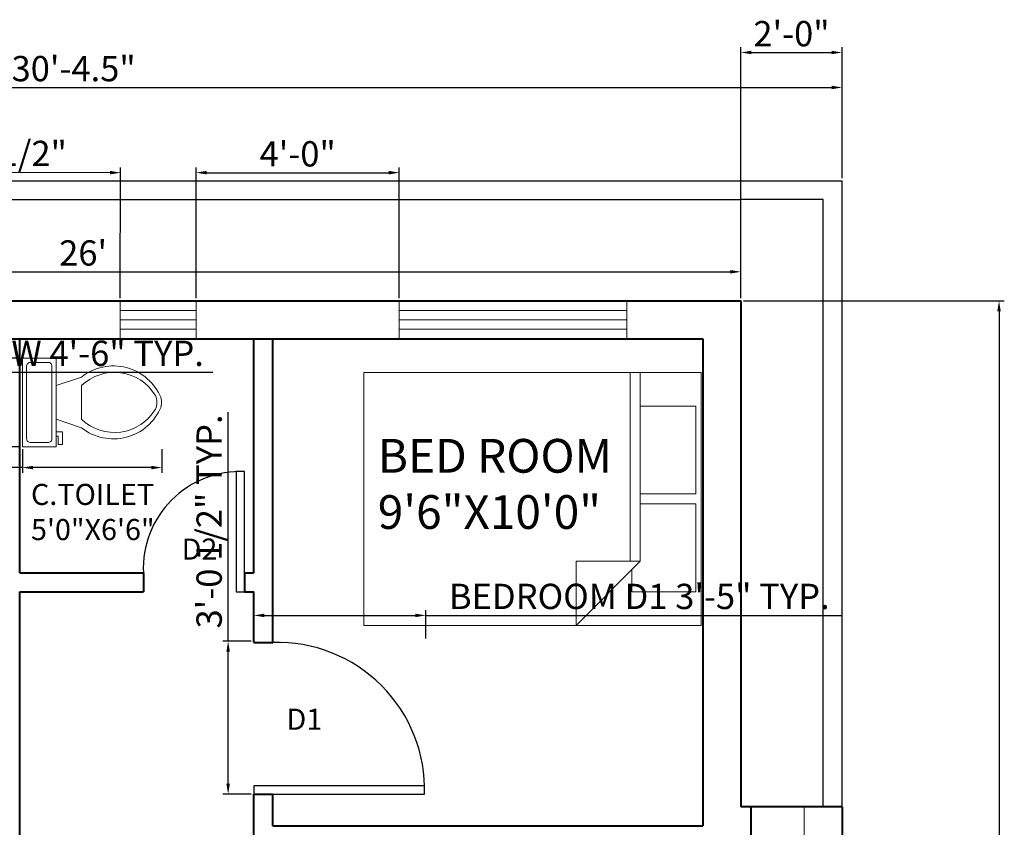
# Model space of a CAD drawing. Units: inches. Extents: x 459864 to 460310, y 324185 to 324787.
# Tile 112 of 112: x 460076 to 460310, y 324591 to 324782. Entities that reach past the tile are written whole.
import ezdxf

# ---------------------------------------------------------------- set-up
doc = ezdxf.new("R2010")
doc.units = ezdxf.units.IN
doc.linetypes.add('ACAD_ISO02W100', pattern=[15, 12, -3])
for name, color, linetype, lineweight in [('A-ANNO-DIMS', 2, 'Continuous', 18), ('A-ANNO-TEXT', 7, 'Continuous', 18), ('A-AREA-IDEN', 7, 'Continuous', 25), ('A-DOOR', 3, 'Continuous', 25), ('A-FLOR-FIXT', 9, 'Continuous', 18), ('A-FURN', 8, 'Continuous', 18), ('A-GLAZ', 4, 'Continuous', 18), ('A-WALL', 7, 'Continuous', 40), ('A-WALL-OVHD', 7, 'ACAD_ISO02W100', 18), ('C-PROP', 7, 'Continuous', 30)]:
    doc.layers.add(name, color=color, linetype=linetype, lineweight=lineweight)
doc.styles.get("Standard").update_dxf_attribs({"font": 'arial.ttf'})
doc.dimstyles.new('ISO-25', dxfattribs={"dimtxt": 6, "dimasz": 2.5, "dimexe": 1.25, "dimexo": 0.625, "dimtad": 1, "dimdec": 1, "dimlunit": 3, "dimtxsty": 'Standard', "dimcen": 2.5, "dimadec": 0, "dimazin": 0, "dimtfac": 1, "dimtdec": 1, "dimtmove": 0, "dimatfit": 3, "dimfxl": 1, "dimarcsym": 0})

# ---------------------------------------------------------------- blocks, each defined once
blk = doc.blocks.new('Window - Wood Frame 36 in. Wide plan')
for p, q in [((0, 6), (0, 0)), ((36, 6), (36, 0)), ((0, 4.5), (36, 4.5)), ((0, 3), (36, 3)), ((0, 1.5), (36, 1.5))]:
    blk.add_line(p, q)
blk = doc.blocks.new('Toilet - top')
for p, q in [((9.5, -6), (9.5, -2)), ((-10, -8.5), (-8, -8.5)), ((-10, -9.5), (-10, -8.5)), ((-8, -8.5), (-8, -8)), ((-7, -8), (-7, -9.5)), ((-4, -8), (-6, -14)), ((4, -8), (6, -14)), ((-7, -9.5), (-10, -9.5)), ((4, -14), (-4, -14))]:
    blk.add_line(p, q)
blk.add_lwpolyline([(10.5, -8), (10.5, 0), (-10.5, 0), (-10.5, -8)], close=True)
for points in [[(-9.5, -2), (-9.5, -6)], [(8.5, -1), (-8.5, -1)], [(-8.5, -7), (8.5, -7)]]:
    blk.add_lwpolyline(points)
for centre, radius, start, end in [((-8.62, -1.88), 0.884, 81.8699, 188.1301), ((8.62, -1.88), 0.884, 351.8699, 98.1301), ((-8.62, -6.12), 0.884, 171.8699, 278.1301), ((8.62, -6.12), 0.884, 261.8699, 8.1301), ((3.52, -21.58), 12.17, 141.4691, 247.9714), ((4.2, -21.82), 11.33, 136.3677, 238.9468), ((-3.52, -21.58), 12.17, 292.0284, 38.5307), ((-4.2, -21.82), 11.33, 301.053, 43.6321), ((0, -27.88), 4, 245.7318, 294.2682), ((0, -29), 4, 254.8605, 285.1395)]:
    blk.add_arc(centre, radius, start, end)
blk = doc.blocks.new('Bed - Queen')
for p, q in [((0, -80.00003), (0, 0)), ((0, 0), (59.99999, 0)), ((59.99999, 0), (59.99999, -80.00003)), ((7.99999, -1.2), (28.79998, -1.2)), ((7.99999, -14.4), (7.99999, -1.2)), ((28.79998, -1.2), (28.79998, -14.4)), ((31.19999, -1.2), (51.99999, -1.2)), ((31.19999, -14.4), (31.19999, -1.2)), ((51.99999, -1.2), (51.99999, -16.4)), ((0, -14.4), (44.8, -14.4)), ((59.99999, -29.6), (44.8, -14.4)), ((44.8, -14.4), (44.8, -29.6)), ((44.8, -16.8), (0, -16.8)), ((51.99999, -16.4), (46.79936, -16.4)), ((44.8, -29.6), (59.99999, -29.6)), ((59.99999, -80.00003), (0, -80.00003))]:
    blk.add_line(p, q)
blk = doc.blocks.new('*D19')
at = {"layer": 'A-ANNO-DIMS', "color": 0, "lineweight": -2, "transparency": 16777216}
for p, q in [((459935.11, 324716.11), (459935.11, 324723.62)), ((459937.61, 324722.37), (460244.61, 324722.37)), ((460247.11, 324716.11), (460247.11, 324723.62))]:
    blk.add_line(p, q, dxfattribs=at)
at = {"layer": 'A-ANNO-DIMS', "color": 0, "transparency": 16777216}
for points in [[(459937.61, 324722.79), (459937.61, 324721.96), (459935.11, 324722.37)], [(460244.61, 324722.79), (460244.61, 324721.96), (460247.11, 324722.37)]]:
    blk.add_solid(points, dxfattribs=at)
at = {"layer": 'Defpoints', "color": 0, "transparency": 16777216}
for p in [(460247.11, 324722.37), (459935.11, 324715.48), (460247.11, 324715.48)]:
    blk.add_point(p, dxfattribs=at)
at = {"layer": 'A-ANNO-DIMS', "color": 0, "transparency": 16777216, "insert": (460091.11, 324726.06), "char_height": 6, "attachment_point": 5}
blk.add_mtext("26'", dxfattribs=at)
blk = doc.blocks.new('*D20')
at = {"layer": 'A-ANNO-DIMS', "color": 0, "lineweight": -2, "transparency": 16777216}
for p, q in [((459906.61, 324744.61), (459906.61, 324767.34)), ((459909.11, 324766.09), (460268.61, 324766.09)), ((460271.11, 324744.61), (460271.11, 324767.34))]:
    blk.add_line(p, q, dxfattribs=at)
at = {"layer": 'A-ANNO-DIMS', "color": 0, "transparency": 16777216}
for points in [[(459909.11, 324766.5), (459909.11, 324765.67), (459906.61, 324766.09)], [(460268.61, 324766.5), (460268.61, 324765.67), (460271.11, 324766.09)]]:
    blk.add_solid(points, dxfattribs=at)
at = {"layer": 'Defpoints', "color": 0, "transparency": 16777216}
for p in [(460271.11, 324766.09), (459906.61, 324743.98), (460271.11, 324743.98)]:
    blk.add_point(p, dxfattribs=at)
at = {"layer": 'A-ANNO-DIMS', "color": 0, "transparency": 16777216, "insert": (460088.86, 324769.78), "char_height": 6, "attachment_point": 5}
blk.add_mtext('30\'-4.5"', dxfattribs=at)
blk = doc.blocks.new('*D21')
at = {"layer": 'A-ANNO-DIMS', "color": 0, "lineweight": -2, "transparency": 16777216}
for p, q in [((460247.74, 324715.48), (460309.58, 324715.48)), ((460308.33, 324712.98), (460308.33, 324285.98)), ((460247.74, 324283.48), (460309.58, 324283.48))]:
    blk.add_line(p, q, dxfattribs=at)
at = {"layer": 'A-ANNO-DIMS', "color": 0, "transparency": 16777216}
for points in [[(460307.91, 324712.98), (460308.75, 324712.98), (460308.33, 324715.48)], [(460307.91, 324285.98), (460308.75, 324285.98), (460308.33, 324283.48)]]:
    blk.add_solid(points, dxfattribs=at)
at = {"layer": 'Defpoints', "color": 0, "transparency": 16777216}
for p in [(460247.11, 324715.48), (460247.11, 324283.48), (460308.33, 324283.48)]:
    blk.add_point(p, dxfattribs=at)
at = {"layer": 'A-ANNO-DIMS', "color": 0, "transparency": 16777216, "insert": (460304.64, 324499.48), "char_height": 6, "attachment_point": 5, "rotation": 90}
blk.add_mtext("36'", dxfattribs=at)
blk = doc.blocks.new('DOOR-SWING-36IN')
for p, q in [((40.5, 2), (0, 2)), ((0, 2), (0, 0)), ((40.5, 0), (40.5, 2)), ((4.5, 0), (40.5, 0))]:
    blk.add_line(p, q)
blk.add_arc((5.5, 1), 35.01, 358.3634, 91.6366)
blk = doc.blocks.new('*D24')
at = {"layer": 'A-ANNO-DIMS', "color": 0, "lineweight": -2, "transparency": 16777216}
for p, q in [((459988.23, 324706.02), (459988.23, 324697.29)), ((460042.23, 324706.02), (460042.23, 324697.29)), ((459990.73, 324698.54), (460039.73, 324698.54)), ((460042.23, 324698.54), (460121.9, 324698.54))]:
    blk.add_line(p, q, dxfattribs=at)
at = {"layer": 'A-ANNO-DIMS', "color": 0, "transparency": 16777216}
for points in [[(459990.73, 324698.96), (459990.73, 324698.13), (459988.23, 324698.54)], [(460039.73, 324698.96), (460039.73, 324698.13), (460042.23, 324698.54)]]:
    blk.add_solid(points, dxfattribs=at)
at = {"layer": 'Defpoints', "color": 0, "transparency": 16777216}
for p in [(459988.23, 324706.64), (460042.23, 324706.64), (460042.23, 324698.54)]:
    blk.add_point(p, dxfattribs=at)
at = {"layer": 'A-ANNO-DIMS', "color": 0, "transparency": 16777216, "insert": (460083.32, 324702.27), "char_height": 6, "attachment_point": 5}
blk.add_mtext('WINDOW 4\'-6" TYP.', dxfattribs=at)
blk = doc.blocks.new('*D30')
at = {"layer": 'A-ANNO-DIMS', "color": 0, "lineweight": -2, "transparency": 16777216}
for p, q in [((460076.72, 324680.27), (460076.72, 324674.69)), ((460109.77, 324680.27), (460109.77, 324674.69)), ((460076.72, 324675.94), (460019.86, 324675.94)), ((460107.27, 324675.94), (460079.22, 324675.94))]:
    blk.add_line(p, q, dxfattribs=at)
at = {"layer": 'A-ANNO-DIMS', "color": 0, "transparency": 16777216}
for points in [[(460079.22, 324676.36), (460079.22, 324675.52), (460076.72, 324675.94)], [(460107.27, 324676.36), (460107.27, 324675.52), (460109.77, 324675.94)]]:
    blk.add_solid(points, dxfattribs=at)
at = {"layer": 'Defpoints', "color": 0, "transparency": 16777216}
for p in [(460076.72, 324680.9), (460109.77, 324680.9), (460076.72, 324675.94)]:
    blk.add_point(p, dxfattribs=at)
at = {"layer": 'A-ANNO-DIMS', "color": 0, "transparency": 16777216, "insert": (460047.04, 324679.67), "char_height": 6, "attachment_point": 5}
blk.add_mtext('WC 2\'-9" TYP.', dxfattribs=at)
blk = doc.blocks.new('*D31')
at = {"layer": 'A-ANNO-DIMS', "color": 0, "lineweight": -2, "transparency": 16777216}
for p, q in [((460071.76, 324701.9), (460071.76, 324741.66)), ((460076.09, 324701.9), (460070.51, 324701.9)), ((460071.76, 324683.4), (460071.76, 324699.4)), ((460076.09, 324680.9), (460070.51, 324680.9))]:
    blk.add_line(p, q, dxfattribs=at)
at = {"layer": 'A-ANNO-DIMS', "color": 0, "transparency": 16777216}
for points in [[(460071.35, 324699.4), (460072.18, 324699.4), (460071.76, 324701.9)], [(460071.35, 324683.4), (460072.18, 324683.4), (460071.76, 324680.9)]]:
    blk.add_solid(points, dxfattribs=at)
at = {"layer": 'Defpoints', "color": 0, "transparency": 16777216}
for p in [(460071.76, 324701.9), (460076.72, 324701.9), (460076.72, 324680.9)]:
    blk.add_point(p, dxfattribs=at)
at = {"layer": 'A-ANNO-DIMS', "color": 0, "transparency": 16777216, "insert": (460068.07, 324723.03), "char_height": 6, "attachment_point": 5, "rotation": 90}
blk.add_mtext('1\'-9" TYP.', dxfattribs=at)
blk = doc.blocks.new('*D38')
at = {"layer": 'A-ANNO-DIMS', "color": 0, "lineweight": -2, "transparency": 16777216}
for p, q in [((460131.61, 324635.39), (460131.61, 324642.13)), ((460172.39, 324635.39), (460172.39, 324642.13)), ((460134.11, 324640.88), (460169.89, 324640.88)), ((460172.39, 324640.88), (460271.13, 324640.88))]:
    blk.add_line(p, q, dxfattribs=at)
at = {"layer": 'A-ANNO-DIMS', "color": 0, "transparency": 16777216}
for points in [[(460134.11, 324641.3), (460134.11, 324640.46), (460131.61, 324640.88)], [(460169.89, 324641.3), (460169.89, 324640.46), (460172.39, 324640.88)]]:
    blk.add_solid(points, dxfattribs=at)
at = {"layer": 'Defpoints', "color": 0, "transparency": 16777216}
for p in [(460172.39, 324640.88), (460131.61, 324634.76), (460172.39, 324634.76)]:
    blk.add_point(p, dxfattribs=at)
at = {"layer": 'A-ANNO-DIMS', "color": 0, "transparency": 16777216, "insert": (460223.01, 324644.61), "char_height": 6, "attachment_point": 5}
blk.add_mtext('BEDROOM D1 3\'-5" TYP.', dxfattribs=at)
blk = doc.blocks.new('*D39')
at = {"layer": 'A-ANNO-DIMS', "color": 0, "lineweight": -2, "transparency": 16777216}
for p, q in [((460125.5, 324634.76), (460125.5, 324689.06)), ((460130.99, 324634.76), (460124.25, 324634.76)), ((460125.5, 324600.99), (460125.5, 324632.26)), ((460130.99, 324598.49), (460124.25, 324598.49))]:
    blk.add_line(p, q, dxfattribs=at)
at = {"layer": 'A-ANNO-DIMS', "color": 0, "transparency": 16777216}
for points in [[(460125.08, 324632.26), (460125.92, 324632.26), (460125.5, 324634.76)], [(460125.08, 324600.99), (460125.92, 324600.99), (460125.5, 324598.49)]]:
    blk.add_solid(points, dxfattribs=at)
at = {"layer": 'Defpoints', "color": 0, "transparency": 16777216}
for p in [(460125.5, 324634.76), (460131.61, 324634.76), (460131.61, 324598.49)]:
    blk.add_point(p, dxfattribs=at)
at = {"layer": 'A-ANNO-DIMS', "color": 0, "transparency": 16777216, "insert": (460121.77, 324663.16), "char_height": 6, "attachment_point": 5, "rotation": 90}
blk.add_mtext('3\'-0 1/2" TYP.', dxfattribs=at)
blk = doc.blocks.new('*D57')
at = {"layer": 'A-ANNO-DIMS', "color": 0, "lineweight": -2, "transparency": 16777216}
for p, q in [((460042.23, 324716.27), (460042.32, 324747.29)), ((460099.91, 324716.11), (460100, 324747.13)), ((460044.81, 324746.04), (460097.5, 324745.89))]:
    blk.add_line(p, q, dxfattribs=at)
at = {"layer": 'A-ANNO-DIMS', "color": 0, "transparency": 16777216}
for points in [[(460044.81, 324746.45), (460044.81, 324745.62), (460042.31, 324746.04)], [(460097.5, 324746.31), (460097.49, 324745.47), (460100, 324745.88)]]:
    blk.add_solid(points, dxfattribs=at)
at = {"layer": 'Defpoints', "color": 0, "transparency": 16777216}
for p in [(460100, 324745.88), (460042.23, 324715.64), (460099.91, 324715.48)]:
    blk.add_point(p, dxfattribs=at)
at = {"layer": 'A-ANNO-DIMS', "color": 0, "transparency": 16777216, "insert": (460071.16, 324749.69), "char_height": 6, "attachment_point": 5, "rotation": 359.8413}
blk.add_mtext('4\'-9 1/2"', dxfattribs=at)
blk = doc.blocks.new('*D58')
at = {"layer": 'A-ANNO-DIMS', "color": 0, "lineweight": -2, "transparency": 16777216}
for p, q in [((460117.91, 324716.11), (460117.91, 324747.13)), ((460166.09, 324716.11), (460166.09, 324747.13)), ((460120.41, 324745.88), (460163.59, 324745.88))]:
    blk.add_line(p, q, dxfattribs=at)
at = {"layer": 'A-ANNO-DIMS', "color": 0, "transparency": 16777216}
for points in [[(460120.41, 324746.3), (460120.41, 324745.47), (460117.91, 324745.88)], [(460163.59, 324746.3), (460163.59, 324745.47), (460166.09, 324745.88)]]:
    blk.add_solid(points, dxfattribs=at)
at = {"layer": 'Defpoints', "color": 0, "transparency": 16777216}
for p in [(460166.09, 324745.88), (460117.91, 324715.48), (460166.09, 324715.48)]:
    blk.add_point(p, dxfattribs=at)
at = {"layer": 'A-ANNO-DIMS', "color": 0, "transparency": 16777216, "insert": (460142, 324749.57), "char_height": 6, "attachment_point": 5}
blk.add_mtext('4\'-0"', dxfattribs=at)
blk = doc.blocks.new('*D66')
at = {"layer": 'A-ANNO-DIMS', "color": 0, "lineweight": -2, "transparency": 16777216}
for p, q in [((460247.11, 324716.11), (460247.11, 324775.63)), ((460271.11, 324744.61), (460271.11, 324775.63)), ((460249.61, 324774.38), (460268.61, 324774.38))]:
    blk.add_line(p, q, dxfattribs=at)
at = {"layer": 'A-ANNO-DIMS', "color": 0, "transparency": 16777216}
for points in [[(460249.61, 324774.8), (460249.61, 324773.97), (460247.11, 324774.38)], [(460268.61, 324774.8), (460268.61, 324773.97), (460271.11, 324774.38)]]:
    blk.add_solid(points, dxfattribs=at)
at = {"layer": 'Defpoints', "color": 0, "transparency": 16777216}
for p in [(460271.11, 324774.38), (460271.11, 324743.98), (460247.11, 324715.48)]:
    blk.add_point(p, dxfattribs=at)
at = {"layer": 'A-ANNO-DIMS', "color": 0, "transparency": 16777216, "insert": (460259.11, 324778.07), "char_height": 6, "attachment_point": 5}
blk.add_mtext('2\'-0"', dxfattribs=at)

msp = doc.modelspace()

# ---------------------------------------------------------------- linework, layer by layer
at = {"layer": 'A-DOOR'}
for p, q in [((460129.4, 324674.98), (460127.4, 324674.98)), ((460127.4, 324674.98), (460127.4, 324646.48)), ((460129.4, 324650.98), (460129.4, 324674.98)), ((460127.4, 324646.48), (460129.4, 324646.48))]:
    msp.add_line(p, q, dxfattribs=at)
msp.add_arc((460128.4, 324651.98), 23.02, 87.5104, 182.4896, dxfattribs=at)
at = {"layer": 'A-WALL'}
for p, q in [((459935.11, 324715.48), (460247.11, 324715.48)), ((460247.11, 324715.48), (460247.11, 324595.48)), ((459944.11, 324706.48), (460238.11, 324706.48)), ((460076.11, 324650.98), (460076.11, 324706.48)), ((460131.61, 324650.98), (460131.61, 324706.48)), ((460136.11, 324634.49), (460136.11, 324706.48)), ((460238.11, 324706.48), (460238.11, 324590.98)), ((460076.11, 324650.98), (460105.4, 324650.98)), ((460105.4, 324650.98), (460105.4, 324646.48)), ((460129.4, 324650.98), (460129.4, 324646.48)), ((460129.4, 324650.98), (460131.61, 324650.98)), ((460076.11, 324586.48), (460076.11, 324646.48)), ((460076.11, 324646.48), (460105.4, 324646.48)), ((460129.4, 324646.48), (460131.61, 324646.48)), ((460131.61, 324634.49), (460131.61, 324646.48)), ((460131.61, 324634.49), (460136.11, 324634.49)), ((460131.61, 324586.48), (460131.61, 324598.49)), ((460131.61, 324598.49), (460136.11, 324598.49)), ((460136.11, 324590.98), (460136.11, 324598.49)), ((460271.11, 324595.48), (460247.11, 324595.48)), ((460249.48, 324595.48), (460249.48, 324586.48)), ((460271.11, 324595.48), (460271.11, 324466.48)), ((460136.11, 324590.98), (460238.11, 324590.98))]:
    msp.add_line(p, q, dxfattribs=at)
at = {"layer": 'A-WALL-OVHD'}
msp.add_line((460262.11, 324586.48), (460262.11, 324595.48), dxfattribs=at)
at = {"layer": 'C-PROP'}
for p, q in [((459906.61, 324743.98), (460271.11, 324743.98)), ((460271.11, 324595.48), (460271.11, 324743.98)), ((459911.11, 324739.48), (460247.11, 324739.48)), ((460266.61, 324739.48), (460247.11, 324739.48)), ((460266.61, 324595.48), (460266.61, 324739.48))]:
    msp.add_line(p, q, dxfattribs=at)

# ---------------------------------------------------------------- block references
at = {"layer": 'A-DOOR'}
msp.add_blockref('DOOR-SWING-36IN', (460131.61, 324598.49), dxfattribs=at)
at = {"layer": 'A-FLOR-FIXT', "rotation": 90}
msp.add_blockref('Toilet - top', (460076.72, 324691.4), dxfattribs=at)
at = {"layer": 'A-FURN', "rotation": 270}
msp.add_blockref('Bed - Queen', (460237.66, 324698.51), dxfattribs=at)
at = {"layer": 'A-GLAZ', "xscale": 0.5, "yscale": 1.5, "zscale": 1.5, "rotation": 180}
msp.add_blockref('Window - Wood Frame 36 in. Wide plan', (460117.91, 324715.48), dxfattribs=at)
at = {"layer": 'A-GLAZ', "xscale": 1.5, "yscale": 1.5, "zscale": 1.5}
msp.add_blockref('Window - Wood Frame 36 in. Wide plan', (460166.09, 324706.48), dxfattribs=at)

# ---------------------------------------------------------------- texts
at = {"layer": 'A-ANNO-TEXT', "char_height": 5, "attachment_point": 1}
for s, insert in [('D2', (460114.47, 324659.11)), ('D1', (460139.35, 324618.76))]:
    msp.add_mtext(s, dxfattribs=dict(at, insert=insert))
at = {"layer": 'A-AREA-IDEN', "attachment_point": 1}
for s, insert, char_height in [('BED ROOM\\P9\'6"X10\'0"', (460160.99, 324682.73), 8), ('C.TOILET\\P5\'0"X6\'6"', (460078.75, 324672.08), 5)]:
    msp.add_mtext(s, dxfattribs=dict(at, insert=insert, char_height=char_height))

# ---------------------------------------------------------------- dimensions: what is measured, and where the dimension line sits
at = {"layer": 'A-ANNO-DIMS'}
for base, p1, p2, override, picture, middle in [((460271.11, 324774.38), (460247.11, 324715.48), (460271.11, 324743.98), {"dimdec": 1, "dimlfac": 1, "dimrnd": 0, "dimzin": 1, "dimdsep": 46, "dimlunit": 4, "dimfrac": 2}, '*D66', (460259.11, 324778.07)), ((460271.11, 324766.09), (459906.61, 324743.98), (460271.11, 324743.98), {"dimclrd": 0, "dimclre": 0, "dimclrt": 0}, '*D20', (460088.86, 324769.78)), ((460166.09, 324745.88), (460117.91, 324715.48), (460166.09, 324715.48), {"dimdec": 1, "dimlfac": 1, "dimrnd": 0, "dimzin": 1, "dimdsep": 46, "dimlunit": 4, "dimfrac": 2}, '*D58', (460142, 324749.57)), ((460247.11, 324722.37), (459935.11, 324715.48), (460247.11, 324715.48), {"dimclrd": 0, "dimclre": 0, "dimclrt": 0}, '*D19', (460091.11, 324726.06))]:
    dim = msp.add_linear_dim(base=base, p1=p1, p2=p2, dimstyle='ISO-25', override=override, dxfattribs=at)
    dim.commit()
    dim.dimension.update_dxf_attribs({"geometry": picture, "text_midpoint": middle})
for base, p1, p2, angle, override, picture, middle in [((460100, 324745.88), (460042.23, 324715.64), (460099.91, 324715.48), 359.8413, {"dimdec": 1, "dimlfac": 1, "dimrnd": 0, "dimzin": 1, "dimdsep": 46, "dimlunit": 4, "dimfrac": 2}, '*D57', (460071.16, 324749.69)), ((460308.33, 324283.48), (460247.11, 324715.48), (460247.11, 324283.48), 90, {"dimclrd": 0, "dimclre": 0, "dimclrt": 0}, '*D21', (460304.64, 324499.48))]:
    dim = msp.add_linear_dim(base=base, p1=p1, p2=p2, angle=angle, dimstyle='ISO-25', override=override, dxfattribs=at)
    dim.commit()
    dim.dimension.update_dxf_attribs({"geometry": picture, "text_midpoint": middle})
for base, p1, p2, angle, text, picture, middle in [((460071.76, 324701.9), (460076.72, 324680.9), (460076.72, 324701.9), 90, '<> TYP.', '*D31', (460068.07, 324723.03)), ((460076.72, 324675.9408), (460109.7662, 324680.8977), (460076.72, 324680.8977), 180, 'WC <> TYP.', '*D30', (460047.0391, 324679.6681)), ((460125.5, 324634.76), (460131.61, 324598.49), (460131.61, 324634.76), 90, '<> TYP.', '*D39', (460121.77, 324663.16))]:
    dim = msp.add_linear_dim(base=base, p1=p1, p2=p2, angle=angle, text=text, dimstyle='ISO-25', override={"dimdec": 1, "dimlfac": 1, "dimrnd": 0, "dimzin": 1, "dimdsep": 46, "dimlunit": 4, "dimfrac": 2}, dxfattribs=at)
    dim.commit()
    dim.dimension.update_dxf_attribs({"geometry": picture, "text_midpoint": middle})
for base, p1, p2, text, picture, middle in [((460042.23, 324698.54), (459988.23, 324706.64), (460042.23, 324706.64), 'WINDOW <> TYP.', '*D24', (460083.32, 324702.27)), ((460172.39, 324640.88), (460131.61, 324634.76), (460172.39, 324634.76), 'BEDROOM D1 <> TYP.', '*D38', (460223.01, 324644.61))]:
    dim = msp.add_linear_dim(base=base, p1=p1, p2=p2, text=text, dimstyle='ISO-25', override={"dimdec": 1, "dimlfac": 1, "dimrnd": 0, "dimzin": 1, "dimdsep": 46, "dimlunit": 4, "dimfrac": 2}, dxfattribs=at)
    dim.commit()
    dim.dimension.update_dxf_attribs({"geometry": picture, "text_midpoint": middle})

doc.saveas('drawing.dxf')
